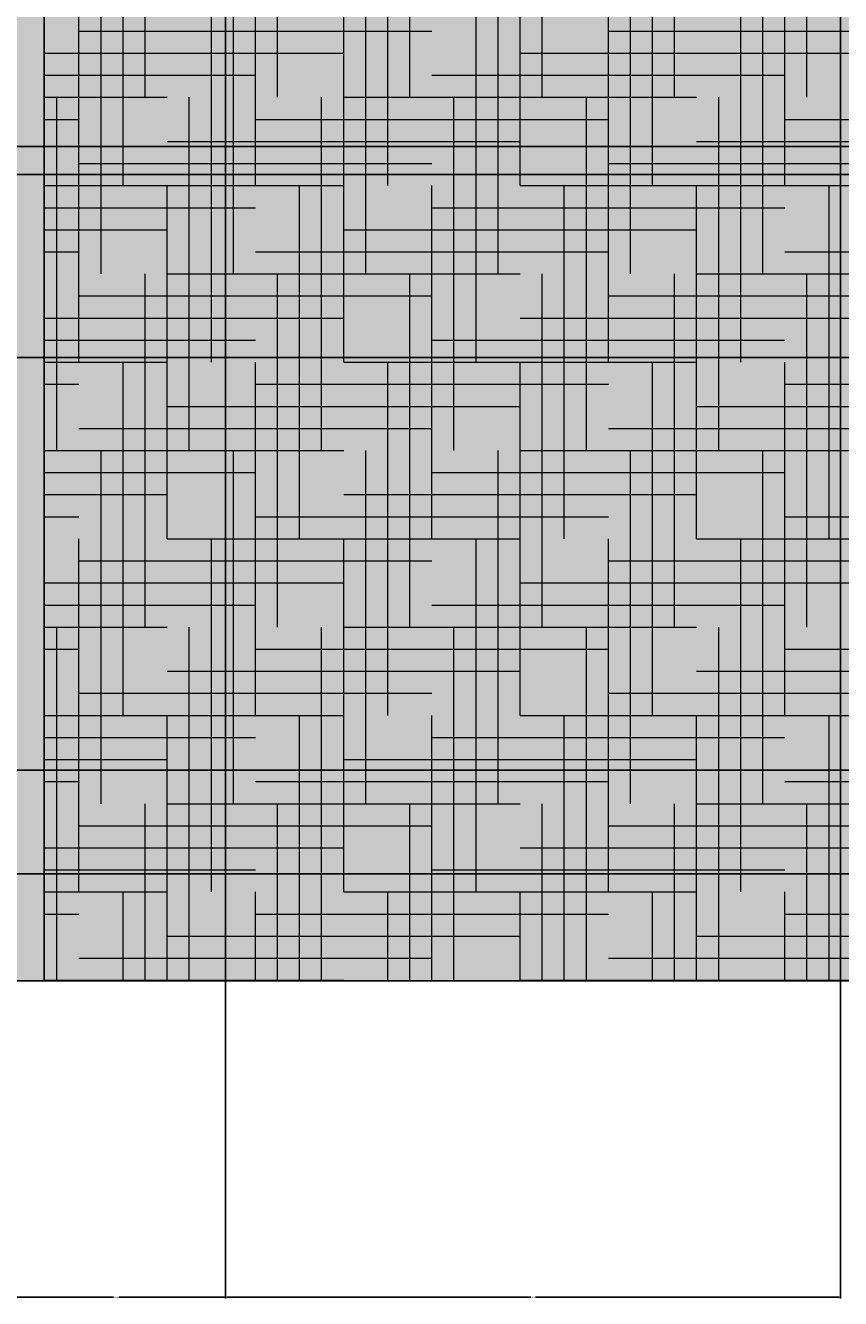
# Model space of a CAD drawing. Units: inches. Extents: x 3024 to 4744, y 1110 to 2100.
# Tile 8 of 29: x 3332 to 3450, y 1110 to 1293. Entities that reach past the tile are written whole.
import ezdxf

# ---------------------------------------------------------------- set-up
doc = ezdxf.new("R2010")
doc.units = ezdxf.units.IN
for name, color, linetype, lineweight in [('A-ANNO-DIMS', 2, 'Continuous', 18), ('A-ELEV', 7, 'Continuous', 25), ('A-ELEV-PATT', 252, 'Continuous', 13)]:
    doc.layers.add(name, color=color, linetype=linetype, lineweight=lineweight)
doc.styles.get("Standard").update_dxf_attribs({"font": 'arial.ttf'})
doc.dimstyles.get("Standard").update_dxf_attribs({"dimtxt": 0.18, "dimasz": 0.18, "dimexe": 0.18, "dimexo": 0.0625, "dimgap": 0.09, "dimtad": 0, "dimtih": 1, "dimtoh": 1, "dimdec": 1, "dimzin": 0, "dimdsep": 46, "dimlunit": 3, "dimtxsty": 'Standard', "dimcen": 0.09, "dimadec": 0, "dimazin": 0, "dimtfac": 1, "dimtdec": 1, "dimtofl": 0, "dimtmove": 0, "dimatfit": 3, "dimfxl": 1, "dimtolj": 1, "dimtzin": 0, "dimarcsym": 0})

# ---------------------------------------------------------------- blocks, each defined once
blk = doc.blocks.new('*D56')
at = {"layer": 'A-ANNO-DIMS', "color": 0, "lineweight": -2, "transparency": 16777216}
for p, q in [((3361.22, 1329.46), (3361.22, 1109.93)), ((3329.7, 1155.55), (3329.7, 1109.93)), ((3329.88, 1110.11), (3345.07, 1110.11)), ((3361.04, 1110.11), (3345.86, 1110.11))]:
    blk.add_line(p, q, dxfattribs=at)
at = {"layer": 'A-ANNO-DIMS', "color": 0, "transparency": 16777216}
for points in [[(3329.88, 1110.14), (3329.88, 1110.08), (3329.7, 1110.11)], [(3361.04, 1110.14), (3361.04, 1110.08), (3361.22, 1110.11)]]:
    blk.add_solid(points, dxfattribs=at)
at = {"layer": 'Defpoints', "color": 0, "transparency": 16777216}
for p in [(3361.22, 1329.52), (3329.7, 1155.61), (3361.22, 1110.11)]:
    blk.add_point(p, dxfattribs=at)
at = {"layer": 'A-ANNO-DIMS', "color": 0, "transparency": 16777216, "insert": (3345.46, 1110.11), "char_height": 0.18, "attachment_point": 5}
blk.add_mtext('\\A1;31.52', dxfattribs=at)
blk = doc.blocks.new('*D57')
at = {"layer": 'A-ANNO-DIMS', "color": 0, "lineweight": -2, "transparency": 16777216}
for p, q in [((3361.22, 1329.46), (3361.22, 1109.93)), ((3449.72, 1329.46), (3449.72, 1109.93)), ((3361.4, 1110.11), (3405.15, 1110.11)), ((3449.54, 1110.11), (3405.8, 1110.11))]:
    blk.add_line(p, q, dxfattribs=at)
at = {"layer": 'A-ANNO-DIMS', "color": 0, "transparency": 16777216}
for points in [[(3361.4, 1110.14), (3361.4, 1110.08), (3361.22, 1110.11)], [(3449.54, 1110.14), (3449.54, 1110.08), (3449.72, 1110.11)]]:
    blk.add_solid(points, dxfattribs=at)
at = {"layer": 'Defpoints', "color": 0, "transparency": 16777216}
for p in [(3361.22, 1329.52), (3449.72, 1329.52), (3449.72, 1110.11)]:
    blk.add_point(p, dxfattribs=at)
at = {"layer": 'A-ANNO-DIMS', "color": 0, "transparency": 16777216, "insert": (3405.47, 1110.11), "char_height": 0.18, "attachment_point": 5}
blk.add_mtext('\\A1;88.5', dxfattribs=at)
blk = doc.blocks.new('*D64')
at = {"layer": 'A-ANNO-DIMS', "color": 0, "lineweight": -2, "transparency": 16777216}
for p, q in [((3069.79, 1241.5), (3069.79, 2100.44)), ((3741.15, 1241.5), (3741.15, 2100.44)), ((3069.97, 2100.26), (3405.08, 2100.26)), ((3740.97, 2100.26), (3405.87, 2100.26))]:
    blk.add_line(p, q, dxfattribs=at)
at = {"layer": 'A-ANNO-DIMS', "color": 0, "transparency": 16777216}
for points in [[(3069.97, 2100.29), (3069.97, 2100.23), (3069.79, 2100.26)], [(3740.97, 2100.29), (3740.97, 2100.23), (3741.15, 2100.26)]]:
    blk.add_solid(points, dxfattribs=at)
at = {"layer": 'Defpoints', "color": 0, "transparency": 16777216}
for p in [(3741.15, 2100.26), (3069.79, 1241.43), (3741.15, 1241.43)]:
    blk.add_point(p, dxfattribs=at)
at = {"layer": 'A-ANNO-DIMS', "color": 0, "transparency": 16777216, "insert": (3405.47, 2100.26), "char_height": 0.18, "attachment_point": 5}
blk.add_mtext('\\A1;671.4', dxfattribs=at)
blk = doc.blocks.new('*D120')
at = {"layer": 'A-ANNO-DIMS', "color": 0, "lineweight": -2, "transparency": 16777216}
for p, q in [((3270.45, 1271.61), (3786.83, 1271.61)), ((3786.65, 1271.43), (3786.65, 1221.5)), ((3786.65, 1171.2), (3786.65, 1221.14)), ((3274.45, 1171.02), (3786.83, 1171.02))]:
    blk.add_line(p, q, dxfattribs=at)
at = {"layer": 'A-ANNO-DIMS', "color": 0, "transparency": 16777216}
for points in [[(3786.62, 1271.43), (3786.68, 1271.43), (3786.65, 1271.61)], [(3786.62, 1171.2), (3786.68, 1171.2), (3786.65, 1171.02)]]:
    blk.add_solid(points, dxfattribs=at)
at = {"layer": 'Defpoints', "color": 0, "transparency": 16777216}
for p in [(3270.39, 1271.61), (3786.65, 1271.61), (3274.39, 1171.02)]:
    blk.add_point(p, dxfattribs=at)
at = {"layer": 'A-ANNO-DIMS', "color": 0, "transparency": 16777216, "insert": (3786.65, 1221.32), "char_height": 0.18, "attachment_point": 5}
blk.add_mtext('\\A1;100.59', dxfattribs=at)
blk = doc.blocks.new('*D121')
at = {"layer": 'A-ANNO-DIMS', "color": 0, "lineweight": -2, "transparency": 16777216}
for p, q in [((3274.45, 1275.61), (3786.83, 1275.61)), ((3786.65, 1275.43), (3786.65, 1273.79)), ((3786.65, 1271.79), (3786.65, 1273.43)), ((3270.45, 1271.61), (3786.83, 1271.61))]:
    blk.add_line(p, q, dxfattribs=at)
at = {"layer": 'A-ANNO-DIMS', "color": 0, "transparency": 16777216}
for points in [[(3786.62, 1275.43), (3786.68, 1275.43), (3786.65, 1275.61)], [(3786.62, 1271.79), (3786.68, 1271.79), (3786.65, 1271.61)]]:
    blk.add_solid(points, dxfattribs=at)
at = {"layer": 'Defpoints', "color": 0, "transparency": 16777216}
for p in [(3274.39, 1275.61), (3786.65, 1275.61), (3270.39, 1271.61)]:
    blk.add_point(p, dxfattribs=at)
at = {"layer": 'A-ANNO-DIMS', "color": 0, "transparency": 16777216, "insert": (3786.65, 1273.61), "char_height": 0.18, "attachment_point": 5}
blk.add_mtext('\\A1;4.00', dxfattribs=at)
blk = doc.blocks.new('*D122')
at = {"layer": 'A-ANNO-DIMS', "color": 0, "lineweight": -2, "transparency": 16777216}
for p, q in [((3228.45, 1185.95), (3786.83, 1185.95)), ((3786.65, 1185.77), (3786.65, 1178.67)), ((3786.65, 1171.2), (3786.65, 1178.31)), ((3270.45, 1171.02), (3786.83, 1171.02))]:
    blk.add_line(p, q, dxfattribs=at)
at = {"layer": 'A-ANNO-DIMS', "color": 0, "transparency": 16777216}
for points in [[(3786.62, 1185.77), (3786.68, 1185.77), (3786.65, 1185.95)], [(3786.62, 1171.2), (3786.68, 1171.2), (3786.65, 1171.02)]]:
    blk.add_solid(points, dxfattribs=at)
at = {"layer": 'Defpoints', "color": 0, "transparency": 16777216}
for p in [(3228.39, 1185.95), (3270.39, 1171.02), (3786.65, 1171.02)]:
    blk.add_point(p, dxfattribs=at)
at = {"layer": 'A-ANNO-DIMS', "color": 0, "transparency": 16777216, "insert": (3786.65, 1178.49), "char_height": 0.18, "attachment_point": 5}
blk.add_mtext('\\A1;14.928', dxfattribs=at)
blk = doc.blocks.new('*D123')
at = {"layer": 'A-ANNO-DIMS', "color": 0, "lineweight": -2, "transparency": 16777216}
for p, q in [((3228.45, 1245.27), (3786.83, 1245.27)), ((3786.65, 1245.09), (3786.65, 1215.79)), ((3786.65, 1186.13), (3786.65, 1215.43)), ((3228.45, 1185.95), (3786.83, 1185.95))]:
    blk.add_line(p, q, dxfattribs=at)
at = {"layer": 'A-ANNO-DIMS', "color": 0, "transparency": 16777216}
for points in [[(3786.62, 1245.09), (3786.68, 1245.09), (3786.65, 1245.27)], [(3786.62, 1186.13), (3786.68, 1186.13), (3786.65, 1185.95)]]:
    blk.add_solid(points, dxfattribs=at)
at = {"layer": 'Defpoints', "color": 0, "transparency": 16777216}
for p in [(3228.39, 1245.27), (3786.65, 1245.27), (3228.39, 1185.95)]:
    blk.add_point(p, dxfattribs=at)
at = {"layer": 'A-ANNO-DIMS', "color": 0, "transparency": 16777216, "insert": (3786.65, 1215.61), "char_height": 0.18, "attachment_point": 5}
blk.add_mtext('\\A1;59.32', dxfattribs=at)

msp = doc.modelspace()

# ---------------------------------------------------------------- hatches: boundary and pattern name
at = {"layer": 'A-ELEV-PATT'}
h = msp.add_hatch(color=256, dxfattribs=at)
h.dxf.hatch_style = 1
h.paths.add_polyline_path([(3335.1044, 2043.5286), (3329.7033, 2043.5286), (3329.7033, 1155.6112), (3335.1044, 1155.6112)])
h.paths.add_polyline_path([(3481.2411, 2043.5286), (3335.1044, 2043.5286), (3335.1044, 1155.6112), (3481.2411, 1155.6112)])
h.paths.add_polyline_path([(3449.7202, 1329.5246), (3361.2242, 1329.5246), (3361.2242, 1436.6064), (3449.7202, 1436.6064)], flags=16)
h.paths.add_polyline_path([(3445.7202, 1333.5246), (3365.2242, 1333.5246), (3365.2242, 1432.6064), (3445.7202, 1432.6064)], flags=0)
h.paths.add_polyline_path([(3449.7202, 1455.5246), (3361.2242, 1455.5246), (3361.2242, 1562.6064), (3449.7202, 1562.6064)], flags=16)
h.paths.add_polyline_path([(3445.7202, 1459.5246), (3365.2242, 1459.5246), (3365.2242, 1558.6064), (3445.7202, 1558.6064)], flags=0)
h.paths.add_polyline_path([(3449.7202, 1581.5246), (3361.2242, 1581.5246), (3361.2242, 1688.6064), (3449.7202, 1688.6064)], flags=16)
h.paths.add_polyline_path([(3445.7202, 1585.5246), (3365.2242, 1585.5246), (3365.2242, 1684.6064), (3445.7202, 1684.6064)], flags=0)
h.paths.add_polyline_path([(3449.7202, 1707.5246), (3361.2242, 1707.5246), (3361.2242, 1814.6064), (3449.7202, 1814.6064)], flags=16)
h.paths.add_polyline_path([(3445.7202, 1711.5246), (3365.2242, 1711.5246), (3365.2242, 1810.6064), (3445.7202, 1810.6064)], flags=0)
h.paths.add_polyline_path([(3449.7202, 1833.5246), (3361.2242, 1833.5246), (3361.2242, 1940.6064), (3449.7202, 1940.6064)], flags=16)
h.paths.add_polyline_path([(3445.7202, 1837.5246), (3365.2242, 1837.5246), (3365.2242, 1936.6064), (3445.7202, 1936.6064)], flags=0)
h = msp.add_hatch(color=256, dxfattribs=at)
h.dxf.hatch_style = 1
h.paths.add_polyline_path([(3475.84, 2043.5286), (3335.1044, 2043.5286), (3335.1044, 1155.6112), (3475.84, 1155.6112)])
h.paths.add_polyline_path([(3449.7202, 1940.6064), (3449.7202, 1833.5246), (3361.2242, 1833.5246), (3361.2242, 1940.6064)], flags=16)
h.paths.add_polyline_path([(3445.7202, 1936.6064), (3445.7202, 1837.5246), (3365.2242, 1837.5246), (3365.2242, 1936.6064)], flags=0)
h.paths.add_polyline_path([(3449.7202, 1814.6064), (3449.7202, 1707.5246), (3361.2242, 1707.5246), (3361.2242, 1814.6064)], flags=16)
h.paths.add_polyline_path([(3445.7202, 1810.6064), (3445.7202, 1711.5246), (3365.2242, 1711.5246), (3365.2242, 1810.6064)], flags=0)
h.paths.add_polyline_path([(3449.7202, 1688.6064), (3449.7202, 1581.5246), (3361.2242, 1581.5246), (3361.2242, 1688.6064)], flags=16)
h.paths.add_polyline_path([(3445.7202, 1684.6064), (3445.7202, 1585.5246), (3365.2242, 1585.5246), (3365.2242, 1684.6064)], flags=0)
h.paths.add_polyline_path([(3449.7202, 1562.6064), (3449.7202, 1455.5246), (3361.2242, 1455.5246), (3361.2242, 1562.6064)], flags=16)
h.paths.add_polyline_path([(3445.7202, 1558.6064), (3445.7202, 1459.5246), (3365.2242, 1459.5246), (3365.2242, 1558.6064)], flags=0)
h.paths.add_polyline_path([(3449.7202, 1436.6064), (3449.7202, 1329.5246), (3361.2242, 1329.5246), (3361.2242, 1436.6064)], flags=16)
h.paths.add_polyline_path([(3445.7202, 1432.6064), (3445.7202, 1333.5246), (3365.2242, 1333.5246), (3365.2242, 1432.6064)], flags=0)
h = msp.add_hatch(dxfattribs=at)
h.set_pattern_fill('HOUND', color=256, scale=2)
h.paths.add_polyline_path([(3475.84, 2043.5286), (3335.1044, 2043.5286), (3335.1044, 1155.6112), (3475.84, 1155.6112)])
h.paths.add_polyline_path([(3449.7202, 1940.6064), (3449.7202, 1833.5246), (3361.2242, 1833.5246), (3361.2242, 1940.6064)], flags=16)
h.paths.add_polyline_path([(3445.7202, 1936.6064), (3445.7202, 1837.5246), (3365.2242, 1837.5246), (3365.2242, 1936.6064)], flags=0)
h.paths.add_polyline_path([(3449.7202, 1814.6064), (3449.7202, 1707.5246), (3361.2242, 1707.5246), (3361.2242, 1814.6064)], flags=16)
h.paths.add_polyline_path([(3445.7202, 1810.6064), (3445.7202, 1711.5246), (3365.2242, 1711.5246), (3365.2242, 1810.6064)], flags=0)
h.paths.add_polyline_path([(3449.7202, 1688.6064), (3449.7202, 1581.5246), (3361.2242, 1581.5246), (3361.2242, 1688.6064)], flags=16)
h.paths.add_polyline_path([(3445.7202, 1684.6064), (3445.7202, 1585.5246), (3365.2242, 1585.5246), (3365.2242, 1684.6064)], flags=0)
h.paths.add_polyline_path([(3449.7202, 1562.6064), (3449.7202, 1455.5246), (3361.2242, 1455.5246), (3361.2242, 1562.6064)], flags=16)
h.paths.add_polyline_path([(3445.7202, 1558.6064), (3445.7202, 1459.5246), (3365.2242, 1459.5246), (3365.2242, 1558.6064)], flags=0)
h.paths.add_polyline_path([(3449.7202, 1436.6064), (3449.7202, 1329.5246), (3361.2242, 1329.5246), (3361.2242, 1436.6064)], flags=16)
h.paths.add_polyline_path([(3445.7202, 1432.6064), (3445.7202, 1333.5246), (3365.2242, 1333.5246), (3365.2242, 1432.6064)], flags=0)
h = msp.add_hatch(dxfattribs=at)
h.set_pattern_fill('ANSI38', color=256, scale=2)
h.paths.add_polyline_path([(3101.9647, 1168.0828), (3103.2358, 1169.5534), (3069.7937, 1169.5534), (3069.7937, 1155.6112), (3101.9647, 1155.6112)])
h.paths.add_polyline_path([(3115.5754, 1168.0828), (3101.9647, 1168.0828), (3101.9647, 1155.6112), (3105.4722, 1155.6112), (3115.5754, 1155.6112)])
h.paths.add_polyline_path([(3118.1176, 1171.0239), (3104.5069, 1171.0239), (3101.9647, 1168.0828), (3115.5754, 1168.0828)])
h.paths.add_polyline_path([(3329.7033, 1171.0239), (3256.7794, 1171.0239, -0.21182003), (3255.8005, 1171.0239), (3249.6327, 1171.0239, -0.21182003), (3248.6539, 1171.0239), (3195.8947, 1171.0239, -0.21182003), (3194.9159, 1171.0239), (3188.7481, 1171.0239, -0.21182003), (3187.7692, 1171.0239), (3118.1176, 1171.0239), (3115.5754, 1168.0828), (3115.5754, 1155.6112), (3329.7033, 1155.6112)])
h.paths.add_polyline_path([(3741.1507, 1169.5534), (3735.4075, 1169.5534), (3705.4722, 1169.5534), (3705.4722, 1155.6112), (3741.1507, 1155.6112)])

# ---------------------------------------------------------------- linework, layer by layer
at = {"layer": 'A-ELEV'}
msp.add_line((3105.4722, 1155.6112), (3705.4722, 1155.6112), dxfattribs=at)
msp.add_line((3105.4722, 1155.6112), (3705.4722, 1155.6112), dxfattribs=at)
for points in [[(3481.2411, 1155.6112), (3329.7033, 1155.6112), (3329.7033, 2043.5286), (3481.2411, 2043.5286)], [(3329.7033, 2043.5286), (3335.1044, 2043.5286), (3335.1044, 1155.6112), (3329.7033, 1155.6112)], [(3481.2411, 1155.6112), (3329.7033, 1155.6112), (3329.7033, 2043.5286), (3481.2411, 2043.5286)], [(3329.7033, 2043.5286), (3335.1044, 2043.5286), (3335.1044, 1155.6112), (3329.7033, 1155.6112)]]:
    msp.add_lwpolyline(points, close=True, dxfattribs=at)

# ---------------------------------------------------------------- dimensions: what is measured, and where the dimension line sits
at = {"layer": 'A-ANNO-DIMS'}
for base, p1, p2, override, picture, middle in [((3741.1507, 2100.2584), (3069.7937, 1241.4341), (3741.1507, 1241.4341), {"dimdec": 1, "dimlfac": 1, "dimrnd": 0, "dimzin": 0, "dimdsep": 46, "dimlunit": 2}, '*D64', (3405.4722, 2100.2584)), ((3361.2242, 1110.1112), (3329.7033, 1155.6112), (3361.2242, 1329.5246), {"dimdec": 2, "dimlfac": 1, "dimrnd": 0, "dimzin": 0, "dimdsep": 46, "dimlunit": 2}, '*D56', (3345.4638, 1110.1112)), ((3449.7202, 1110.1112), (3361.2242, 1329.5246), (3449.7202, 1329.5246), {"dimdec": 1, "dimlfac": 1, "dimrnd": 0, "dimzin": 0, "dimdsep": 46, "dimlunit": 2}, '*D57', (3405.4722, 1110.1112))]:
    dim = msp.add_linear_dim(base=base, p1=p1, p2=p2, dimstyle='Standard', override=override, dxfattribs=at)
    dim.commit()
    dim.dimension.update_dxf_attribs({"geometry": picture, "text_midpoint": middle})
for base, p1, p2, override, picture, middle in [((3786.6507, 1275.6112), (3270.3877, 1271.6112), (3274.3877, 1275.6112), {"dimdec": 2, "dimlfac": 1, "dimrnd": 0, "dimzin": 0, "dimdsep": 46, "dimlunit": 2}, '*D121', (3786.6507, 1273.6112)), ((3786.6507, 1271.6112), (3274.3877, 1171.0239), (3270.3877, 1271.6112), {"dimdec": 2, "dimlfac": 1, "dimrnd": 0, "dimzin": 0, "dimdsep": 46, "dimlunit": 2}, '*D120', (3786.6507, 1221.3176)), ((3786.6507, 1245.2708), (3228.3856, 1185.9515), (3228.3856, 1245.2708), {"dimdec": 2, "dimlfac": 1, "dimrnd": 0, "dimzin": 0, "dimdsep": 46, "dimlunit": 2}, '*D123', (3786.6507, 1215.6112)), ((3786.6507, 1171.0239), (3228.3856, 1185.9515), (3270.3877, 1171.0239), {"dimdec": 3, "dimlfac": 1, "dimrnd": 0, "dimzin": 0, "dimdsep": 46, "dimlunit": 2}, '*D122', (3786.6507, 1178.4877))]:
    dim = msp.add_linear_dim(base=base, p1=p1, p2=p2, angle=90, dimstyle='Standard', override=override, dxfattribs=at)
    dim.commit()
    dim.dimension.update_dxf_attribs({"geometry": picture, "text_midpoint": middle})

doc.saveas('drawing.dxf')
